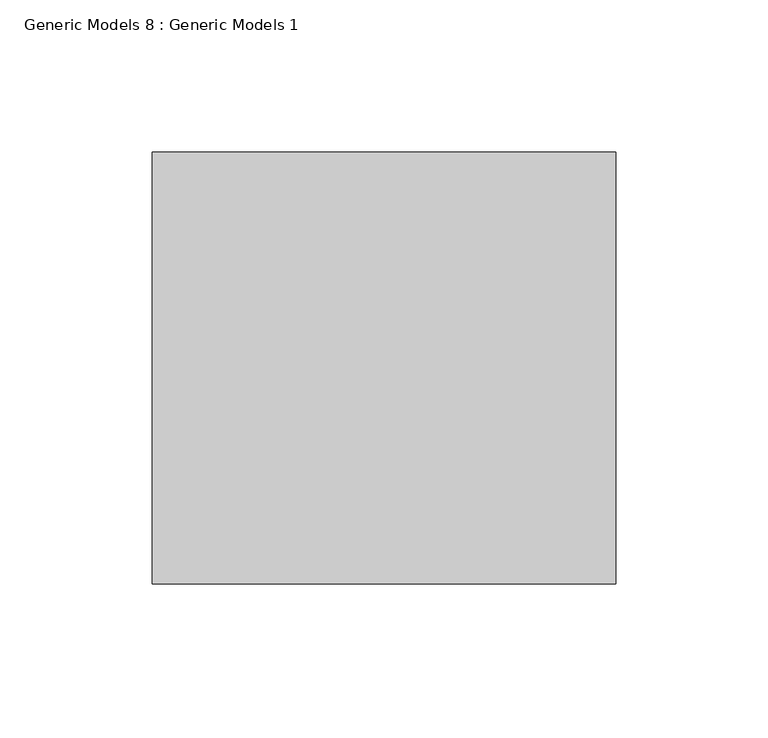
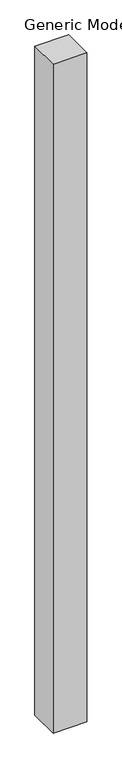
"""IFC4 building model written with IfcOpenShell, lengths in millimetres: proxy geometry, Generic Models 8 : Generic Models 1."""

from ifc_helpers import new_model, si_unit, origin, origin_with_axes, place, context, project, spatial, polyline, outline, extrude, source, transform, mapped, element, save


def generic_models_8_generic_models_1_2d490598(model_context):
    return source(origin(), model_context, "Body", "SweptSolid", [
        extrude(outline(polyline([(-11757.069475, -5471.7273102), (-11604.669475, -5471.7273102), (-11604.669475, -5613.7098142), (-11757.069475, -5613.7098142), (-11757.069475, -5471.7273102)])), origin_with_axes(), (0.0, 0.0, 1.0), 3200.4),
    ])


if __name__ == "__main__":
    model = new_model("IFC4")
    model_context = context("Model", 3, world=origin())
    ifc_project = project(units=[si_unit("LENGTHUNIT", "METRE", prefix="MILLI")], contexts=[model_context])
    site = spatial("IfcSite", under=ifc_project)
    building = spatial("IfcBuilding", under=site)
    placement = place(None, origin())
    generic_models_8_generic_models_1_shape = generic_models_8_generic_models_1_2d490598(model_context)
    element("IfcBuildingElementProxy", 1, Name="Generic Models 8 : Generic Models 1", ObjectType="Generic Models 8 : Generic Models 1", at=placement, inside=building, context=model_context, shape_type="MappedRepresentation", body=[
        mapped(generic_models_8_generic_models_1_shape, transform((0.0, 0.0, 0.0), x_axis=(1.0, 0.0, 0.0), y_axis=(0.0, 1.0, 0.0), z_axis=(0.0, 0.0, 1.0))),
    ])
    save(model, "model.ifc")
